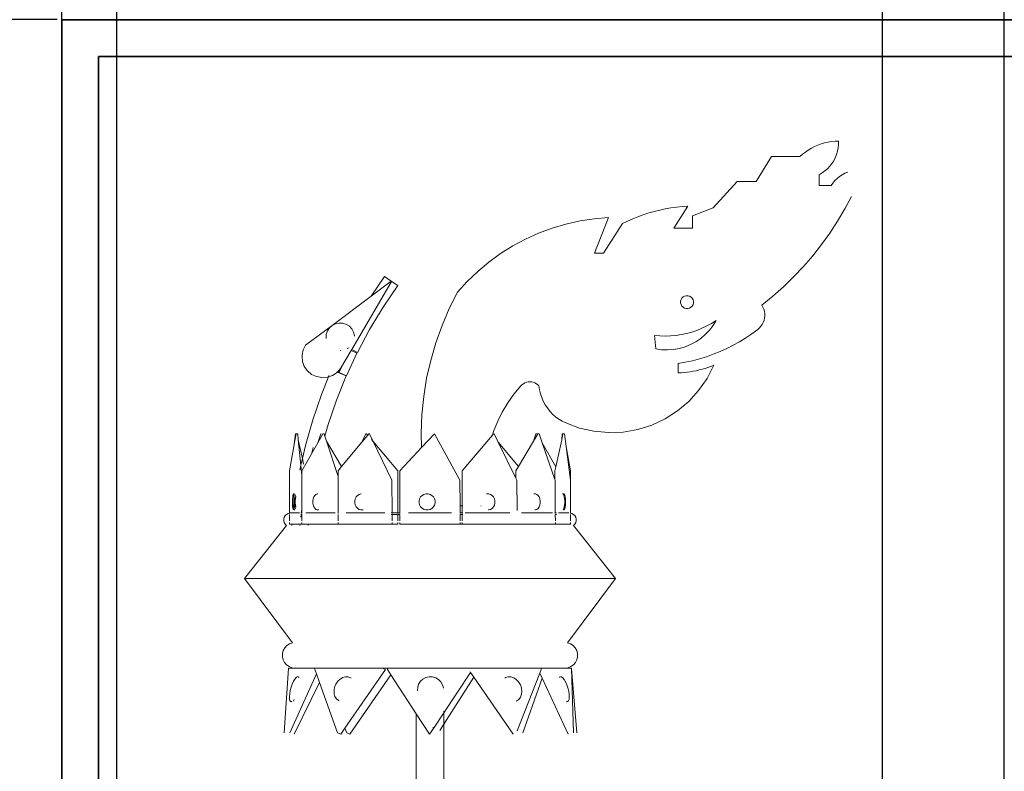
# Model space of a CAD drawing. Units: millimetres. Extents: x 446512 to 447461, y 70395 to 70610.
# Tile 12 of 39: x 446686 to 446699.43, y 70483.13 to 70493.38. Entities that reach past the tile are written whole.
import ezdxf

# ---------------------------------------------------------------- set-up
doc = ezdxf.new("R2010")
doc.units = ezdxf.units.MM
for name, color, linetype, lineweight in [('A-ANNO-DIMS', 2, 'Continuous', 18), ('A-CONS', 9, 'Continuous', 13), ('A-FURN', 7, 'Continuous', 35), ('A-FURN-DECO', 8, 'Continuous', 13)]:
    doc.layers.add(name, color=color, linetype=linetype, lineweight=lineweight)
doc.styles.get("Standard").update_dxf_attribs({"font": 'arial.ttf'})
doc.dimstyles.get("Standard").update_dxf_attribs({"dimtxt": 0.18, "dimasz": 0.18, "dimexe": 0.18, "dimexo": 0.0625, "dimgap": 0.09, "dimtad": 0, "dimtih": 1, "dimtoh": 1, "dimdec": 4, "dimzin": 0, "dimdsep": 46, "dimtxsty": 'Standard', "dimcen": 0.09, "dimadec": 0, "dimazin": 0, "dimtfac": 1, "dimtdec": 4, "dimtofl": 0, "dimtmove": 0, "dimatfit": 3, "dimfxl": 1, "dimtolj": 1, "dimtzin": 0, "dimarcsym": 0})

# ---------------------------------------------------------------- blocks, each defined once
blk = doc.blocks.new('*D21')
at = {"layer": 'A-ANNO-DIMS', "color": 0, "lineweight": -2, "transparency": 16777216}
for p, q in [((446686.51, 70493.382), (446678.043, 70493.382)), ((446678.223, 70493.202), (446678.223, 70483.563)), ((446678.223, 70473.562), (446678.223, 70483.2)), ((446686.51, 70473.382), (446678.043, 70473.382))]:
    blk.add_line(p, q, dxfattribs=at)
at = {"layer": 'A-ANNO-DIMS', "color": 0, "transparency": 16777216}
for points in [[(446678.193, 70493.202), (446678.253, 70493.202), (446678.223, 70493.382)], [(446678.193, 70473.562), (446678.253, 70473.562), (446678.223, 70473.382)]]:
    blk.add_solid(points, dxfattribs=at)
at = {"layer": 'Defpoints', "color": 0, "transparency": 16777216}
for p in [(446678.223, 70493.382), (446686.573, 70493.382), (446686.573, 70473.382)]:
    blk.add_point(p, dxfattribs=at)
at = {"layer": 'A-ANNO-DIMS', "color": 0, "transparency": 16777216, "insert": (446678.223, 70483.382), "char_height": 0.18, "attachment_point": 5}
blk.add_mtext('\\A1;20', dxfattribs=at)
blk = doc.blocks.new('*D37')
at = {"layer": 'A-ANNO-DIMS', "color": 0, "lineweight": -2, "transparency": 16777216}
for p, q in [((446686.572846, 70433.44405), (446686.572846, 70578.17492)), ((446687.323552, 70428.838404), (446687.323552, 70578.17492)), ((446686.392846, 70577.99492), (446686.212846, 70577.99492)), ((446687.503552, 70577.99492), (446687.683552, 70577.99492))]:
    blk.add_line(p, q, dxfattribs=at)
at = {"layer": 'A-ANNO-DIMS', "color": 0, "transparency": 16777216}
for points in [[(446686.392846, 70578.02492), (446686.392846, 70577.96492), (446686.572846, 70577.99492)], [(446687.503552, 70578.02492), (446687.503552, 70577.96492), (446687.323552, 70577.99492)]]:
    blk.add_solid(points, dxfattribs=at)
at = {"layer": 'Defpoints', "color": 0, "transparency": 16777216}
for p in [(446687.323552, 70577.99492), (446686.572846, 70433.38155), (446687.323552, 70428.775904)]:
    blk.add_point(p, dxfattribs=at)
at = {"layer": 'A-ANNO-DIMS', "color": 0, "transparency": 16777216, "insert": (446686.948199, 70577.99492), "char_height": 0.18, "attachment_point": 5}
blk.add_mtext('\\A1;0.75', dxfattribs=at)
blk = doc.blocks.new('*D38')
at = {"layer": 'A-ANNO-DIMS', "color": 0, "lineweight": -2, "transparency": 16777216}
for p, q in [((446687.323552, 70428.838404), (446687.323552, 70578.17492)), ((446697.765686, 70428.838404), (446697.765686, 70578.17492)), ((446687.503552, 70577.99492), (446692.090383, 70577.99492)), ((446697.585686, 70577.99492), (446692.998855, 70577.99492))]:
    blk.add_line(p, q, dxfattribs=at)
at = {"layer": 'A-ANNO-DIMS', "color": 0, "transparency": 16777216}
for points in [[(446687.503552, 70578.02492), (446687.503552, 70577.96492), (446687.323552, 70577.99492)], [(446697.585686, 70578.02492), (446697.585686, 70577.96492), (446697.765686, 70577.99492)]]:
    blk.add_solid(points, dxfattribs=at)
at = {"layer": 'Defpoints', "color": 0, "transparency": 16777216}
for p in [(446697.765686, 70577.99492), (446687.323552, 70428.775904), (446697.765686, 70428.775904)]:
    blk.add_point(p, dxfattribs=at)
at = {"layer": 'A-ANNO-DIMS', "color": 0, "transparency": 16777216, "insert": (446692.544619, 70577.99492), "char_height": 0.18, "attachment_point": 5}
blk.add_mtext('\\A1;10.442', dxfattribs=at)
blk = doc.blocks.new('*D39')
at = {"layer": 'A-ANNO-DIMS', "color": 0, "lineweight": -2, "transparency": 16777216}
for p, q in [((446697.766, 70428.838), (446697.766, 70578.175)), ((446699.429, 70433.444), (446699.429, 70578.175)), ((446697.946, 70577.995), (446698.212, 70577.995)), ((446699.249, 70577.995), (446698.982, 70577.995))]:
    blk.add_line(p, q, dxfattribs=at)
at = {"layer": 'A-ANNO-DIMS', "color": 0, "transparency": 16777216}
for points in [[(446697.946, 70578.025), (446697.946, 70577.965), (446697.766, 70577.995)], [(446699.249, 70578.025), (446699.249, 70577.965), (446699.429, 70577.995)]]:
    blk.add_solid(points, dxfattribs=at)
at = {"layer": 'Defpoints', "color": 0, "transparency": 16777216}
for p in [(446699.429, 70577.995), (446699.429, 70433.382), (446697.766, 70428.776)]:
    blk.add_point(p, dxfattribs=at)
at = {"layer": 'A-ANNO-DIMS', "color": 0, "transparency": 16777216, "insert": (446698.597, 70577.995), "char_height": 0.18, "attachment_point": 5}
blk.add_mtext('\\A1;1.663', dxfattribs=at)

msp = doc.modelspace()

# ---------------------------------------------------------------- linework, layer by layer
at = {"layer": 'A-CONS'}
msp.add_point((446686.5728, 70493.3815), dxfattribs=at)
at = {"layer": 'A-FURN'}
for p, q in [((446686.5728, 70493.3815), (446746.5728, 70493.3815)), ((446686.5728, 70473.3815), (446686.5728, 70493.3815))]:
    msp.add_line(p, q, dxfattribs=at)
for points in [[(446686.5728, 70493.3815), (446729.0084, 70493.3815), (446729.0084, 70473.3815), (446686.5728, 70473.3815)], [(446687.0728, 70492.8815), (446728.5084, 70492.8815), (446728.5084, 70473.8815), (446687.0728, 70473.8815)]]:
    msp.add_lwpolyline(points, close=True, dxfattribs=at)
at = {"layer": 'A-FURN-DECO'}
for p, q in [((446696.7153, 70491.5764), (446696.7552, 70491.6041)), ((446696.7552, 70491.6041), (446696.7968, 70491.6292)), ((446696.7968, 70491.6292), (446696.84, 70491.6515)), ((446696.84, 70491.6515), (446696.8844, 70491.6711)), ((446696.8844, 70491.6711), (446696.9301, 70491.6877)), ((446696.9301, 70491.6877), (446696.9767, 70491.7015)), ((446696.9767, 70491.7015), (446697.024, 70491.7122)), ((446697.024, 70491.7122), (446697.072, 70491.7198)), ((446697.072, 70491.7198), (446697.1204, 70491.7244)), ((446697.1204, 70491.7244), (446697.1689, 70491.7259)), ((446697.1638, 70491.6329), (446697.1547, 70491.5872)), ((446697.1686, 70491.6793), (446697.1638, 70491.6329)), ((446697.1689, 70491.7259), (446697.1686, 70491.6793)), ((446696.0452, 70491.1756), (446696.2545, 70491.5137)), ((446696.2545, 70491.5137), (446696.6411, 70491.5137)), ((446696.6411, 70491.5137), (446696.6772, 70491.5463)), ((446696.6772, 70491.5463), (446696.7153, 70491.5764)), ((446697.1237, 70491.4993), (446697.1021, 70491.458)), ((446697.1413, 70491.5425), (446697.1237, 70491.4993)), ((446697.1547, 70491.5872), (446697.1413, 70491.5425)), ((446697.0155, 70491.3487), (446696.9802, 70491.3182)), ((446697.0478, 70491.3823), (446697.0155, 70491.3487)), ((446697.0767, 70491.4189), (446697.0478, 70491.3823)), ((446697.1021, 70491.458), (446697.0767, 70491.4189)), ((446696.9421, 70491.2912), (446696.9017, 70491.268)), ((446696.9017, 70491.268), (446696.9017, 70491.1188)), ((446696.9802, 70491.3182), (446696.9421, 70491.2912)), ((446697.118, 70491.1867), (446697.148, 70491.2166)), ((446697.148, 70491.2166), (446697.1808, 70491.2435)), ((446697.1808, 70491.2435), (446697.2159, 70491.2671)), ((446697.2159, 70491.2671), (446697.2532, 70491.2872)), ((446697.2532, 70491.2872), (446697.2923, 70491.3036)), ((446695.4573, 70490.8173), (446695.7856, 70491.1756)), ((446695.7856, 70491.1756), (446696.0452, 70491.1756)), ((446696.9017, 70491.1188), (446697.0674, 70491.1188)), ((446697.0674, 70491.1188), (446697.0911, 70491.154)), ((446697.0911, 70491.154), (446697.118, 70491.1867)), ((446697.3425, 70490.9725), (446697.2517, 70490.8013)), ((446694.7284, 70490.7852), (446694.8042, 70490.801)), ((446694.8042, 70490.801), (446694.8805, 70490.8141)), ((446694.8805, 70490.8141), (446694.9573, 70490.8245)), ((446695.1116, 70490.8369), (446694.921, 70490.5393)), ((446694.9573, 70490.8245), (446695.0343, 70490.8321)), ((446695.0343, 70490.8321), (446695.1116, 70490.8369)), ((446695.175, 70490.705), (446695.4573, 70490.8173)), ((446697.2517, 70490.8013), (446697.1532, 70490.6345)), ((446693.6414, 70490.6372), (446693.836, 70490.6671)), ((446693.836, 70490.6671), (446694.0321, 70490.6837)), ((446694.0321, 70490.6837), (446693.8395, 70490.1957)), ((446694.2897, 70490.6344), (446694.3604, 70490.666)), ((446694.3604, 70490.666), (446694.4322, 70490.6951)), ((446694.4322, 70490.6951), (446694.505, 70490.7216)), ((446694.505, 70490.7216), (446694.5787, 70490.7454)), ((446694.5787, 70490.7454), (446694.6532, 70490.7666)), ((446694.6532, 70490.7666), (446694.7284, 70490.7852)), ((446695.175, 70490.5393), (446695.175, 70490.705)), ((446693.0762, 70490.4696), (446693.2607, 70490.5382)), ((446693.2607, 70490.5382), (446693.4494, 70490.5942)), ((446693.4494, 70490.5942), (446693.6414, 70490.6372)), ((446693.961, 70490.1957), (446694.2202, 70490.6003)), ((446694.2202, 70490.6003), (446694.2897, 70490.6344)), ((446694.921, 70490.5393), (446695.175, 70490.5393)), ((446697.1532, 70490.6345), (446697.0475, 70490.4721)), ((446692.8968, 70490.3885), (446693.0762, 70490.4696)), ((446697.0475, 70490.4721), (446696.9346, 70490.3147)), ((446692.5566, 70490.1909), (446692.7233, 70490.2955)), ((446692.7233, 70490.2955), (446692.8968, 70490.3885)), ((446696.9346, 70490.3147), (446696.8148, 70490.1624)), ((446692.3973, 70490.0753), (446692.5566, 70490.1909)), ((446693.8395, 70490.1957), (446693.961, 70490.1957)), ((446696.8148, 70490.1624), (446696.6883, 70490.0156)), ((446692.2463, 70489.9491), (446692.3973, 70490.0753)), ((446696.6883, 70490.0156), (446696.5554, 70489.8746)), ((446690.9762, 70489.8801), (446690.7926, 70489.6121)), ((446691.0674, 70489.8177), (446690.9762, 70489.8801)), ((446692.1042, 70489.8129), (446692.2463, 70489.9491)), ((446696.5554, 70489.8746), (446696.4164, 70489.7397)), ((446691.0674, 70489.8034), (446690.5277, 70488.8832)), ((446691.0674, 70489.8177), (446690.7926, 70489.6121)), ((446690.9564, 70489.4602), (446691.1585, 70489.7553)), ((446691.0674, 70489.8034), (446691.0674, 70489.8177)), ((446691.1585, 70489.7553), (446691.0674, 70489.8177)), ((446691.9716, 70489.6674), (446692.1042, 70489.8129)), ((446696.4164, 70489.7397), (446696.2714, 70489.6111)), ((446690.7926, 70489.6121), (446690.2614, 70489.2121)), ((446691.9716, 70489.6674), (446691.8583, 70489.4434)), ((446695.0198, 70489.5639), (446695.0314, 70489.5838)), ((446695.0314, 70489.5838), (446695.0478, 70489.6001)), ((446695.0478, 70489.6001), (446695.0679, 70489.6115)), ((446695.0679, 70489.6115), (446695.0902, 70489.6174)), ((446695.0902, 70489.6174), (446695.1133, 70489.6172)), ((446695.1133, 70489.6172), (446695.1355, 70489.6112)), ((446695.1355, 70489.6112), (446695.1554, 70489.5995)), ((446695.1554, 70489.5995), (446695.1717, 70489.5831)), ((446696.2714, 70489.6111), (446696.1209, 70489.4891)), ((446690.772, 70489.1572), (446690.9564, 70489.4602)), ((446695.0136, 70489.5186), (446695.0137, 70489.5417)), ((446695.0195, 70489.4963), (446695.0136, 70489.5186)), ((446695.0137, 70489.5417), (446695.0198, 70489.5639)), ((446695.0309, 70489.4763), (446695.0195, 70489.4963)), ((446695.0471, 70489.4599), (446695.0309, 70489.4763)), ((446695.067, 70489.4482), (446695.0471, 70489.4599)), ((446695.1547, 70489.4593), (446695.1347, 70489.4479)), ((446695.1711, 70489.4755), (446695.1547, 70489.4593)), ((446695.1827, 70489.4954), (446695.1711, 70489.4755)), ((446695.1717, 70489.5831), (446695.1831, 70489.5631)), ((446695.1888, 70489.5177), (446695.1827, 70489.4954)), ((446695.1831, 70489.5631), (446695.1889, 70489.5408)), ((446695.1889, 70489.5408), (446695.1888, 70489.5177)), ((446696.1209, 70489.4891), (446696.1363, 70489.4624)), ((446696.1363, 70489.4624), (446696.1482, 70489.4339)), ((446691.8583, 70489.4434), (446691.7591, 70489.2129)), ((446695.0893, 70489.4421), (446695.067, 70489.4482)), ((446695.1124, 70489.442), (446695.0893, 70489.4421)), ((446695.1347, 70489.4479), (446695.1124, 70489.442)), ((446696.1482, 70489.4339), (446696.1565, 70489.4042)), ((446696.1565, 70489.4042), (446696.161, 70489.3736)), ((446696.1617, 70489.3428), (446696.1586, 70489.3121)), ((446696.161, 70489.3736), (446696.1617, 70489.3428)), ((446690.2614, 70489.2121), (446689.8973, 70488.9421)), ((446690.2238, 70489.1795), (446690.2614, 70489.2121)), ((446690.2614, 70489.2121), (446690.3063, 70489.2342)), ((446690.3063, 70489.2342), (446690.3557, 70489.2444)), ((446690.3557, 70489.2444), (446690.4061, 70489.2418)), ((446690.4061, 70489.2418), (446690.4541, 70489.2267)), ((446690.4541, 70489.2267), (446690.4964, 70489.2002)), ((446690.4964, 70489.2002), (446690.5301, 70489.1639)), ((446691.7591, 70489.2129), (446691.6743, 70488.9767)), ((446695.3717, 70489.2046), (446695.3051, 70489.1729)), ((446695.4363, 70489.2402), (446695.3717, 70489.2046)), ((446695.4562, 70489.2103), (446695.4067, 70489.1459)), ((446695.4988, 70489.2795), (446695.4363, 70489.2402)), ((446695.4988, 70489.2795), (446695.4562, 70489.2103)), ((446696.1092, 70489.2002), (446696.0887, 70489.1771)), ((446696.1267, 70489.2256), (446696.1092, 70489.2002)), ((446696.1409, 70489.253), (446696.1267, 70489.2256)), ((446696.1516, 70489.282), (446696.1409, 70489.253)), ((446696.1586, 70489.3121), (446696.1516, 70489.282)), ((446690.1781, 70489.0436), (446690.1807, 70489.0923)), ((446690.1807, 70489.0923), (446690.1964, 70489.1387)), ((446690.1964, 70489.1387), (446690.2238, 70489.1795)), ((446690.5301, 70489.1639), (446690.553, 70489.1205)), ((446690.553, 70489.1205), (446690.5635, 70489.0728)), ((446690.5631, 70489.0659), (446690.5635, 70489.0728)), ((446690.5631, 70489.0659), (446690.5635, 70489.0642)), ((446690.772, 70489.1572), (446690.6043, 70488.8447)), ((446694.7296, 70489.0686), (446694.6561, 70489.0749)), ((446694.6561, 70489.0749), (446694.6742, 70488.8914)), ((446694.8034, 70489.0666), (446694.7296, 70489.0686)), ((446694.8771, 70489.069), (446694.8034, 70489.0666)), ((446694.9506, 70489.0757), (446694.8771, 70489.069)), ((446695.0235, 70489.0868), (446694.9506, 70489.0757)), ((446695.0957, 70489.102), (446695.0235, 70489.0868)), ((446695.1668, 70489.1215), (446695.0957, 70489.102)), ((446695.2367, 70489.1452), (446695.1668, 70489.1215)), ((446695.3051, 70489.1729), (446695.2367, 70489.1452)), ((446695.3506, 70489.0872), (446695.2887, 70489.0346)), ((446695.4067, 70489.1459), (446695.3506, 70489.0872)), ((446695.9853, 70489.0978), (446695.9028, 70489.0422)), ((446696.0655, 70489.1568), (446695.9853, 70489.0978)), ((446696.0887, 70489.1771), (446696.0655, 70489.1568)), ((446689.8973, 70488.9421), (446689.8648, 70488.8771)), ((446690.1785, 70489.0419), (446690.1781, 70489.0436)), ((446690.1781, 70489.035), (446690.1785, 70489.0419)), ((446691.6743, 70488.9767), (446691.6043, 70488.7356)), ((446695.0748, 70488.9198), (446694.9968, 70488.8973)), ((446695.15, 70488.9505), (446695.0748, 70488.9198)), ((446695.2216, 70488.9889), (446695.15, 70488.9505)), ((446695.2887, 70489.0346), (446695.2216, 70488.9889)), ((446695.731, 70488.9416), (446695.6421, 70488.8968)), ((446695.8179, 70488.9901), (446695.731, 70488.9416)), ((446695.9028, 70489.0422), (446695.8179, 70488.9901)), ((446689.8648, 70488.8771), (446689.8508, 70488.8062)), ((446689.8508, 70488.7919), (446689.8508, 70488.8062)), ((446689.8508, 70488.7919), (446689.8563, 70488.7199)), ((446690.3735, 70488.8727), (446690.3696, 70488.8643)), ((446690.52, 70488.8701), (446690.3759, 70488.6244)), ((446690.4548, 70488.5258), (446690.5989, 70488.8331)), ((446690.464, 70488.8963), (446690.473, 70488.8922)), ((446690.4885, 70488.9029), (446690.4822, 70488.906)), ((446690.5277, 70488.8832), (446690.52, 70488.8701)), ((446690.5989, 70488.8331), (446690.52, 70488.8701)), ((446690.5277, 70488.8832), (446690.6043, 70488.8447)), ((446694.7547, 70488.8801), (446694.6742, 70488.8914)), ((446694.8358, 70488.8773), (446694.7547, 70488.8801)), ((446694.9168, 70488.883), (446694.8358, 70488.8773)), ((446694.9968, 70488.8973), (446694.9168, 70488.883)), ((446695.3653, 70488.7853), (446695.2702, 70488.756)), ((446695.4591, 70488.8186), (446695.3653, 70488.7853)), ((446695.5515, 70488.8558), (446695.4591, 70488.8186)), ((446695.6421, 70488.8968), (446695.5515, 70488.8558)), ((446689.8563, 70488.7199), (446689.8809, 70488.6518)), ((446689.8809, 70488.6518), (446689.923, 70488.5921)), ((446690.3917, 70488.6514), (446690.3548, 70488.5727)), ((446691.6043, 70488.7356), (446691.5493, 70488.4908)), ((446695.0767, 70488.7094), (446694.9787, 70488.6923)), ((446694.9787, 70488.6923), (446694.9787, 70488.5652)), ((446695.174, 70488.7307), (446695.0767, 70488.7094)), ((446695.2702, 70488.756), (446695.174, 70488.7307)), ((446695.4649, 70488.6683), (446695.3736, 70488.4897)), ((446695.3869, 70488.6393), (446695.4261, 70488.6532)), ((446695.4261, 70488.6532), (446695.4649, 70488.6683)), ((446689.923, 70488.5921), (446689.9796, 70488.545)), ((446689.9796, 70488.545), (446690.0468, 70488.5136)), ((446690.0468, 70488.5136), (446690.1203, 70488.5001)), ((446690.2103, 70488.5106), (446690.1138, 70488.2721)), ((446690.1948, 70488.5054), (446690.2103, 70488.5106)), ((446690.2103, 70488.5106), (446690.2653, 70488.5292)), ((446690.2169, 70488.5272), (446690.2103, 70488.5106)), ((446690.2653, 70488.5292), (446690.3271, 70488.5698)), ((446690.3208, 70488.1948), (446690.4538, 70488.5236)), ((446690.3223, 70488.5809), (446690.3329, 70488.5763)), ((446690.3271, 70488.5698), (446690.3329, 70488.5763)), ((446690.3371, 70488.581), (446690.3289, 70488.5848)), ((446690.3329, 70488.5763), (446690.3371, 70488.581)), ((446690.3329, 70488.5763), (446690.4538, 70488.5236)), ((446690.3371, 70488.581), (446690.3759, 70488.6244)), ((446690.3371, 70488.581), (446690.4548, 70488.5258)), ((446690.3548, 70488.5727), (446690.3525, 70488.5678)), ((446694.9787, 70488.5652), (446695.0203, 70488.5672)), ((446695.0203, 70488.5672), (446695.0618, 70488.5703)), ((446695.0618, 70488.5703), (446695.1032, 70488.5747)), ((446695.1032, 70488.5747), (446695.1445, 70488.5803)), ((446695.1445, 70488.5803), (446695.1855, 70488.5871)), ((446695.1855, 70488.5871), (446695.2264, 70488.5952)), ((446695.2264, 70488.5952), (446695.267, 70488.6044)), ((446695.267, 70488.6044), (446695.3073, 70488.6149)), ((446695.3073, 70488.6149), (446695.3473, 70488.6265)), ((446695.3473, 70488.6265), (446695.3869, 70488.6393)), ((446690.1203, 70488.5001), (446690.1948, 70488.5054)), ((446691.5493, 70488.4908), (446691.5095, 70488.2429)), ((446692.8329, 70488.3878), (446692.7393, 70488.2755)), ((446692.8497, 70488.4039), (446692.8329, 70488.3878)), ((446692.8685, 70488.4176), (446692.8497, 70488.4039)), ((446692.8891, 70488.4286), (446692.8685, 70488.4176)), ((446692.9111, 70488.4365), (446692.8891, 70488.4286)), ((446692.9339, 70488.4414), (446692.9111, 70488.4365)), ((446692.9571, 70488.443), (446692.9339, 70488.4414)), ((446692.9804, 70488.4414), (446692.9571, 70488.443)), ((446693.0032, 70488.4365), (446692.9804, 70488.4414)), ((446693.0251, 70488.4286), (446693.0032, 70488.4365)), ((446693.0457, 70488.4176), (446693.0251, 70488.4286)), ((446693.0646, 70488.4039), (446693.0457, 70488.4176)), ((446693.0814, 70488.3878), (446693.0646, 70488.4039)), ((446693.0894, 70488.3339), (446693.0814, 70488.3878)), ((446695.3736, 70488.4897), (446695.2594, 70488.3247)), ((446690.1138, 70488.2721), (446689.9949, 70487.9253)), ((446691.5095, 70488.2429), (446691.4851, 70487.9931)), ((446692.7393, 70488.2755), (446692.6548, 70488.1561)), ((446693.1021, 70488.281), (446693.0894, 70488.3339)), ((446693.1193, 70488.2293), (446693.1021, 70488.281)), ((446695.2594, 70488.3247), (446695.1246, 70488.1761)), ((446690.2058, 70487.8593), (446690.3208, 70488.1948)), ((446692.6548, 70488.1561), (446692.58, 70488.0305)), ((446693.141, 70488.1794), (446693.1193, 70488.2293)), ((446693.1669, 70488.1315), (446693.141, 70488.1794)), ((446693.1969, 70488.0861), (446693.1669, 70488.1315)), ((446695.1246, 70488.1761), (446694.9714, 70488.0466)), ((446691.4851, 70487.9931), (446691.4762, 70487.7423)), ((446692.58, 70488.0305), (446692.5154, 70487.8993)), ((446693.2308, 70488.0435), (446693.1969, 70488.0861)), ((446693.2682, 70488.0039), (446693.2308, 70488.0435)), ((446693.3089, 70487.9678), (446693.2682, 70488.0039)), ((446694.9714, 70488.0466), (446694.8024, 70487.9384)), ((446689.9949, 70487.9253), (446689.8949, 70487.5726)), ((446690.1611, 70487.7015), (446690.2058, 70487.8593)), ((446692.5154, 70487.8993), (446692.4613, 70487.7635)), ((446693.3526, 70487.9353), (446693.3089, 70487.9678)), ((446693.399, 70487.9068), (446693.3526, 70487.9353)), ((446693.4476, 70487.8824), (446693.399, 70487.9068)), ((446693.6358, 70487.8127), (446693.4476, 70487.8824)), ((446694.6207, 70487.8534), (446694.4293, 70487.7931)), ((446694.8024, 70487.9384), (446694.6207, 70487.8534)), ((446689.7422, 70487.5943), (446689.7597, 70487.732)), ((446689.7686, 70487.732), (446689.7422, 70487.5943)), ((446689.7686, 70487.732), (446689.7597, 70487.732)), ((446689.7686, 70487.732), (446689.7903, 70487.732)), ((446689.7985, 70487.653), (446689.7903, 70487.732)), ((446690.0658, 70487.6129), (446690.1072, 70487.732)), ((446690.1333, 70487.732), (446690.0658, 70487.6129)), ((446690.1123, 70487.732), (446690.1072, 70487.732)), ((446690.151, 70487.732), (446690.1333, 70487.732)), ((446690.1611, 70487.7015), (446690.151, 70487.732)), ((446690.6667, 70487.6207), (446690.7216, 70487.732)), ((446690.7455, 70487.7153), (446690.6667, 70487.6207)), ((446690.7312, 70487.732), (446690.7216, 70487.732)), ((446690.7312, 70487.732), (446690.7455, 70487.7153)), ((446690.7594, 70487.732), (446690.7455, 70487.7153)), ((446690.7699, 70487.732), (446690.7594, 70487.732)), ((446690.8204, 70487.6273), (446690.7699, 70487.732)), ((446691.4762, 70487.7423), (446691.4814, 70487.5462)), ((446691.6572, 70487.732), (446691.4814, 70487.5462)), ((446692.0025, 70487.1025), (446691.6572, 70487.732)), ((446692.446, 70487.714), (446692.0321, 70487.2307)), ((446692.446, 70487.714), (446692.4417, 70487.7003)), ((446692.4472, 70487.7181), (446692.446, 70487.714)), ((446692.446, 70487.714), (446692.4496, 70487.7096)), ((446692.4613, 70487.7635), (446692.4472, 70487.7181)), ((446692.4591, 70487.732), (446692.4472, 70487.7181)), ((446692.4591, 70487.732), (446692.4687, 70487.732)), ((446692.5236, 70487.6207), (446692.4687, 70487.732)), ((446693.0069, 70487.6333), (446693.0393, 70487.732)), ((446693.0614, 70487.7242), (446693.0069, 70487.6333)), ((446693.0393, 70487.732), (446693.057, 70487.732)), ((446693.057, 70487.732), (446693.0614, 70487.7242)), ((446693.0661, 70487.732), (446693.0614, 70487.7242)), ((446693.0661, 70487.732), (446693.0831, 70487.732)), ((446693.1245, 70487.6129), (446693.0831, 70487.732)), ((446693.3918, 70487.653), (446693.4, 70487.732)), ((446693.4091, 70487.732), (446693.3918, 70487.653)), ((446693.4, 70487.732), (446693.4091, 70487.732)), ((446693.4091, 70487.732), (446693.4306, 70487.732)), ((446693.4306, 70487.732), (446693.4525, 70487.5599)), ((446693.8314, 70487.7684), (446693.6358, 70487.8127)), ((446694.0312, 70487.7502), (446693.8314, 70487.7684)), ((446694.2317, 70487.7585), (446694.0312, 70487.7502)), ((446694.4293, 70487.7931), (446694.2317, 70487.7585)), ((446689.7378, 70487.5599), (446689.7422, 70487.5943)), ((446689.7985, 70487.653), (446689.855, 70487.3957)), ((446689.8346, 70487.3054), (446689.7985, 70487.653)), ((446690.0658, 70487.6129), (446689.849, 70487.2307)), ((446689.8949, 70487.5726), (446689.855, 70487.3957)), ((446690.1834, 70487.6333), (446690.1611, 70487.7015)), ((446690.1834, 70487.6333), (446690.3901, 70487.2886)), ((446690.3419, 70487.1511), (446690.1834, 70487.6333)), ((446690.6667, 70487.6207), (446690.3901, 70487.2886)), ((446690.7961, 70487.6558), (446690.8204, 70487.6273)), ((446690.8204, 70487.6273), (446691.1582, 70487.2307)), ((446691.0736, 70487.1025), (446690.8204, 70487.6273)), ((446692.5236, 70487.6207), (446692.8002, 70487.2886)), ((446692.5236, 70487.6207), (446692.7654, 70487.1306)), ((446693.0069, 70487.6333), (446692.8002, 70487.2886)), ((446693.1245, 70487.6129), (446693.3109, 70487.2842)), ((446693.1245, 70487.6129), (446693.2991, 70487.1102)), ((446693.3918, 70487.653), (446693.3109, 70487.2842)), ((446689.7378, 70487.5599), (446689.6789, 70487.2307)), ((446690.002, 70487.5453), (446689.9851, 70487.4707)), ((446691.4814, 70487.5462), (446691.1826, 70487.2307)), ((446693.4525, 70487.5599), (446693.5114, 70487.2307)), ((446693.5107, 70487.1025), (446693.4525, 70487.5599)), ((446689.8346, 70487.3054), (446689.8197, 70487.2395)), ((446689.855, 70487.3957), (446689.8346, 70487.3054)), ((446689.849, 70487.1659), (446689.8346, 70487.3054)), ((446689.855, 70487.3957), (446689.8713, 70487.3212)), ((446689.6789, 70487.2307), (446689.6807, 70487.1103)), ((446689.849, 70487.2307), (446689.849, 70487.1659)), ((446690.3901, 70487.2886), (446690.3419, 70487.2307)), ((446690.3419, 70487.2307), (446690.3419, 70487.1511)), ((446691.1582, 70487.2307), (446691.1582, 70486.6542)), ((446691.1826, 70487.2307), (446691.1826, 70486.6542)), ((446692.0321, 70487.2307), (446692.0321, 70486.7516)), ((446692.8002, 70487.2886), (446692.7654, 70487.2307)), ((446692.7654, 70487.2307), (446692.7654, 70487.1306)), ((446693.3109, 70487.2842), (446693.2991, 70487.2307)), ((446693.2991, 70487.2307), (446693.2991, 70487.1102)), ((446693.5114, 70487.2307), (446693.5107, 70487.1025)), ((446689.6797, 70487.1025), (446689.6788, 70486.6528)), ((446689.6797, 70487.1025), (446689.6807, 70487.1103)), ((446689.849, 70487.1659), (446689.849, 70486.6542)), ((446690.3419, 70487.1511), (446690.3419, 70486.648)), ((446691.0736, 70487.1025), (446691.077, 70486.6542)), ((446692.0025, 70487.1025), (446692.0055, 70486.7514)), ((446692.7793, 70487.1025), (446692.7654, 70487.1306)), ((446692.7793, 70487.1025), (446692.7825, 70486.6881)), ((446693.3018, 70487.1025), (446693.2991, 70487.1102)), ((446693.3018, 70487.1025), (446693.3043, 70486.6542)), ((446693.5107, 70487.1025), (446693.5115, 70486.6528)), ((446689.7257, 70486.8933), (446689.7305, 70486.9077)), ((446689.7305, 70486.9077), (446689.7357, 70486.915)), ((446689.7466, 70486.915), (446689.7357, 70486.915)), ((446689.7366, 70486.8933), (446689.7413, 70486.9077)), ((446689.7413, 70486.9077), (446689.7466, 70486.915)), ((446689.7598, 70486.8998), (446689.757, 70486.8929)), ((446689.7604, 70486.898), (446689.757, 70486.8929)), ((446690.023, 70486.8933), (446690.038, 70486.9077)), ((446690.038, 70486.9077), (446690.0547, 70486.915)), ((446690.0635, 70486.915), (446690.0547, 70486.915)), ((446690.605, 70486.8933), (446690.627, 70486.9077)), ((446690.627, 70486.9077), (446690.6516, 70486.915)), ((446690.6568, 70486.915), (446690.6516, 70486.915)), ((446691.4878, 70486.8933), (446691.5128, 70486.9077)), ((446691.5128, 70486.9077), (446691.5407, 70486.915)), ((446691.5407, 70486.915), (446691.5695, 70486.915)), ((446691.5695, 70486.915), (446691.5973, 70486.9074)), ((446691.5973, 70486.9074), (446691.6223, 70486.8929)), ((446692.3638, 70486.915), (446692.3687, 70486.915)), ((446692.3687, 70486.915), (446692.3946, 70486.915)), ((446692.3946, 70486.915), (446692.4196, 70486.9074)), ((446692.4196, 70486.9074), (446692.4421, 70486.8929)), ((446693.0093, 70486.915), (446693.0179, 70486.915)), ((446693.0179, 70486.915), (446693.0361, 70486.915)), ((446693.0361, 70486.915), (446693.0537, 70486.9074)), ((446693.0537, 70486.9074), (446693.0695, 70486.8929)), ((446693.4036, 70486.915), (446693.4103, 70486.915)), ((446693.4103, 70486.915), (446693.4167, 70486.9074)), ((446693.4103, 70486.915), (446693.4144, 70486.915)), ((446693.4144, 70486.915), (446693.421, 70486.915)), ((446693.4167, 70486.9074), (446693.4225, 70486.8929)), ((446693.421, 70486.915), (446693.4275, 70486.9074)), ((446693.4275, 70486.9074), (446693.4333, 70486.8929)), ((446689.7177, 70486.8202), (446689.7191, 70486.848)), ((446689.7177, 70486.7914), (446689.7177, 70486.8202)), ((446689.7191, 70486.7635), (446689.7177, 70486.7914)), ((446689.7191, 70486.848), (446689.7219, 70486.873)), ((446689.7218, 70486.7385), (446689.7191, 70486.7635)), ((446689.7219, 70486.873), (446689.7257, 70486.8933)), ((446689.7285, 70486.8202), (446689.73, 70486.848)), ((446689.7285, 70486.7914), (446689.7285, 70486.8202)), ((446689.7299, 70486.7635), (446689.7285, 70486.7914)), ((446689.7326, 70486.7385), (446689.7299, 70486.7635)), ((446689.73, 70486.848), (446689.7327, 70486.873)), ((446689.7327, 70486.873), (446689.7366, 70486.8933)), ((446689.7473, 70486.7908), (446689.7365, 70486.718)), ((446689.749, 70486.8475), (446689.7473, 70486.8196)), ((446689.7473, 70486.8196), (446689.7473, 70486.7908)), ((446689.7473, 70486.7908), (446689.7491, 70486.763)), ((446689.7523, 70486.8725), (446689.749, 70486.8475)), ((446689.7528, 70486.8536), (446689.749, 70486.8475)), ((446689.757, 70486.8929), (446689.7523, 70486.8725)), ((446689.7523, 70486.8725), (446689.7528, 70486.8536)), ((446689.7597, 70486.8475), (446689.758, 70486.8196)), ((446689.758, 70486.8196), (446689.7581, 70486.7908)), ((446689.7581, 70486.7908), (446689.7598, 70486.763)), ((446689.7631, 70486.8725), (446689.7597, 70486.8475)), ((446689.7646, 70486.8791), (446689.7631, 70486.8725)), ((446689.9975, 70486.8202), (446690.002, 70486.848)), ((446689.9975, 70486.7914), (446689.9975, 70486.8202)), ((446690.0019, 70486.7635), (446689.9975, 70486.7914)), ((446690.0105, 70486.7385), (446690.0019, 70486.7635)), ((446690.002, 70486.848), (446690.0107, 70486.873)), ((446690.0107, 70486.873), (446690.023, 70486.8933)), ((446690.5676, 70486.7914), (446690.5677, 70486.8202)), ((446690.5741, 70486.7635), (446690.5676, 70486.7914)), ((446690.5677, 70486.8202), (446690.5743, 70486.848)), ((446690.5867, 70486.7385), (446690.5741, 70486.7635)), ((446690.5743, 70486.848), (446690.5871, 70486.873)), ((446690.5871, 70486.873), (446690.605, 70486.8933)), ((446691.4452, 70486.7914), (446691.4453, 70486.8202)), ((446691.4526, 70486.7635), (446691.4452, 70486.7914)), ((446691.4453, 70486.8202), (446691.4528, 70486.848)), ((446691.467, 70486.7385), (446691.4526, 70486.7635)), ((446691.4528, 70486.848), (446691.4673, 70486.873)), ((446691.4673, 70486.873), (446691.4878, 70486.8933)), ((446691.6223, 70486.8929), (446691.6426, 70486.8725)), ((446691.6426, 70486.8725), (446691.6569, 70486.8475)), ((446691.6643, 70486.7908), (446691.6567, 70486.763)), ((446691.6569, 70486.8475), (446691.6643, 70486.8196)), ((446691.6643, 70486.8196), (446691.6643, 70486.7908)), ((446692.4421, 70486.8929), (446692.4604, 70486.8725)), ((446692.4604, 70486.8725), (446692.4733, 70486.8475)), ((446692.4799, 70486.7908), (446692.4731, 70486.763)), ((446692.4733, 70486.8475), (446692.4799, 70486.8196)), ((446692.4799, 70486.8196), (446692.4799, 70486.7908)), ((446693.0695, 70486.8929), (446693.0824, 70486.8725)), ((446693.0824, 70486.8725), (446693.0915, 70486.8475)), ((446693.0961, 70486.7908), (446693.0914, 70486.763)), ((446693.0915, 70486.8475), (446693.0962, 70486.8196)), ((446693.0962, 70486.8196), (446693.0961, 70486.7908)), ((446693.4225, 70486.8929), (446693.4272, 70486.8725)), ((446693.4272, 70486.8725), (446693.4306, 70486.8475)), ((446693.4323, 70486.7908), (446693.4305, 70486.763)), ((446693.4306, 70486.8475), (446693.4323, 70486.8196)), ((446693.4323, 70486.8196), (446693.4323, 70486.7908)), ((446693.4333, 70486.8929), (446693.438, 70486.8725)), ((446693.438, 70486.8725), (446693.4413, 70486.8475)), ((446693.4413, 70486.8475), (446693.443, 70486.8196)), ((446693.443, 70486.7908), (446693.4413, 70486.763)), ((446693.443, 70486.8196), (446693.443, 70486.7908)), ((446689.6198, 70486.6182), (446689.6379, 70486.6357)), ((446689.6379, 70486.6357), (446689.66, 70486.648)), ((446689.66, 70486.648), (446689.6788, 70486.6528)), ((446689.6787, 70486.6357), (446689.6785, 70486.547)), ((446689.6788, 70486.6528), (446689.6844, 70486.6542)), ((446689.6788, 70486.6528), (446689.6788, 70486.648)), ((446689.6844, 70486.6542), (446689.6887, 70486.6542)), ((446689.6844, 70486.6542), (446689.6862, 70486.6542)), ((446689.8138, 70486.6542), (446689.6887, 70486.6542)), ((446689.7256, 70486.718), (446689.7218, 70486.7385)), ((446689.7303, 70486.7036), (446689.7256, 70486.718)), ((446689.7356, 70486.696), (446689.7303, 70486.7036)), ((446689.7365, 70486.718), (446689.7326, 70486.7385)), ((446689.7411, 70486.6959), (446689.7356, 70486.696)), ((446689.7412, 70486.7036), (446689.7365, 70486.718)), ((446689.7465, 70486.696), (446689.7411, 70486.6959)), ((446689.7465, 70486.696), (446689.7412, 70486.7036)), ((446689.7519, 70486.6959), (446689.7465, 70486.696)), ((446689.7491, 70486.763), (446689.7524, 70486.738)), ((446689.7524, 70486.738), (446689.7571, 70486.7177)), ((446689.7571, 70486.7177), (446689.7598, 70486.7112)), ((446689.7598, 70486.763), (446689.7632, 70486.738)), ((446689.7632, 70486.738), (446689.7646, 70486.7318)), ((446689.849, 70486.6542), (446689.8346, 70486.6542)), ((446689.8391, 70486.6357), (446689.8347, 70486.5979)), ((446689.849, 70486.6341), (446689.8347, 70486.6341)), ((446689.849, 70486.7227), (446689.8405, 70486.648)), ((446689.849, 70486.6542), (446689.849, 70486.648)), ((446689.849, 70486.6357), (446689.849, 70486.6341)), ((446689.849, 70486.6341), (446689.849, 70486.547)), ((446690.3002, 70486.6542), (446689.9013, 70486.6542)), ((446690.0227, 70486.718), (446690.0105, 70486.7385)), ((446690.0376, 70486.7036), (446690.0227, 70486.718)), ((446690.0543, 70486.696), (446690.0376, 70486.7036)), ((446690.0716, 70486.6959), (446690.0543, 70486.696)), ((446690.0804, 70486.6959), (446690.0716, 70486.6959)), ((446690.3419, 70486.6357), (446690.3419, 70486.547)), ((446690.4496, 70486.6542), (446690.9806, 70486.6542)), ((446690.6046, 70486.718), (446690.5867, 70486.7385)), ((446690.6266, 70486.7036), (446690.6046, 70486.718)), ((446690.6511, 70486.696), (446690.6266, 70486.7036)), ((446690.6764, 70486.6959), (446690.6511, 70486.696)), ((446690.6817, 70486.6959), (446690.6764, 70486.6959)), ((446691.077, 70486.6542), (446691.0665, 70486.6542)), ((446691.0772, 70486.6341), (446691.0666, 70486.6341)), ((446691.077, 70486.6542), (446691.077, 70486.648)), ((446691.1582, 70486.6542), (446691.077, 70486.6542)), ((446691.0771, 70486.6357), (446691.0772, 70486.6341)), ((446691.0772, 70486.6341), (446691.0778, 70486.547)), ((446691.1582, 70486.6341), (446691.0772, 70486.6341)), ((446691.1582, 70486.6542), (446691.1826, 70486.6542)), ((446691.1582, 70486.6542), (446691.1582, 70486.648)), ((446691.1582, 70486.6357), (446691.1582, 70486.6341)), ((446691.1582, 70486.6341), (446691.1582, 70486.547)), ((446691.1826, 70486.6341), (446691.1582, 70486.6341)), ((446691.1826, 70486.6542), (446691.1826, 70486.648)), ((446691.1826, 70486.6357), (446691.1826, 70486.6341)), ((446691.1826, 70486.6341), (446691.1826, 70486.547)), ((446691.3015, 70486.6542), (446691.8889, 70486.6542)), ((446691.4873, 70486.718), (446691.467, 70486.7385)), ((446691.5122, 70486.7036), (446691.4873, 70486.718)), ((446691.5401, 70486.696), (446691.5122, 70486.7036)), ((446691.5689, 70486.6959), (446691.5401, 70486.696)), ((446691.5968, 70486.7033), (446691.5689, 70486.6959)), ((446691.6218, 70486.7177), (446691.5968, 70486.7033)), ((446691.6422, 70486.738), (446691.6218, 70486.7177)), ((446691.6567, 70486.763), (446691.6422, 70486.738)), ((446692.0321, 70486.7516), (446692.0055, 70486.7514)), ((446692.0055, 70486.7514), (446692.0064, 70486.6542)), ((446692.0064, 70486.6542), (446692.0064, 70486.648)), ((446692.0321, 70486.6542), (446692.0064, 70486.6542)), ((446692.0065, 70486.6357), (446692.0066, 70486.6341)), ((446692.0066, 70486.6341), (446692.0073, 70486.547)), ((446692.0321, 70486.6341), (446692.0066, 70486.6341)), ((446692.0418, 70486.7517), (446692.0321, 70486.7516)), ((446692.0321, 70486.7516), (446692.0321, 70486.6542)), ((446692.0418, 70486.6542), (446692.0321, 70486.6542)), ((446692.0321, 70486.6542), (446692.0321, 70486.648)), ((446692.0321, 70486.6357), (446692.0321, 70486.6341)), ((446692.0418, 70486.6341), (446692.0321, 70486.6341)), ((446692.0321, 70486.6341), (446692.0321, 70486.547)), ((446692.0765, 70486.6542), (446692.6838, 70486.6542)), ((446692.2944, 70486.7539), (446692.2896, 70486.7538)), ((446692.3893, 70486.6959), (446692.3941, 70486.6959)), ((446692.4192, 70486.7033), (446692.3941, 70486.6959)), ((446692.4417, 70486.7177), (446692.4192, 70486.7033)), ((446692.46, 70486.738), (446692.4417, 70486.7177)), ((446692.4731, 70486.763), (446692.46, 70486.738)), ((446693.2678, 70486.6542), (446692.8447, 70486.6542)), ((446693.0272, 70486.6959), (446693.0358, 70486.6959)), ((446693.0534, 70486.7033), (446693.0358, 70486.6959)), ((446693.0692, 70486.7177), (446693.0534, 70486.7033)), ((446693.0822, 70486.738), (446693.0692, 70486.7177)), ((446693.0914, 70486.763), (446693.0822, 70486.738)), ((446693.3206, 70486.6542), (446693.3043, 70486.6542)), ((446693.3043, 70486.6542), (446693.3043, 70486.648)), ((446693.3044, 70486.6357), (446693.3044, 70486.6341)), ((446693.3206, 70486.6341), (446693.3044, 70486.6341)), ((446693.3044, 70486.6341), (446693.3049, 70486.547)), ((446693.349, 70486.6542), (446693.4889, 70486.6542)), ((446693.4166, 70486.7033), (446693.4102, 70486.6959)), ((446693.4102, 70486.6959), (446693.4209, 70486.6959)), ((446693.4224, 70486.7177), (446693.4166, 70486.7033)), ((446693.4274, 70486.7033), (446693.4209, 70486.6959)), ((446693.4272, 70486.738), (446693.4224, 70486.7177)), ((446693.4305, 70486.763), (446693.4272, 70486.738)), ((446693.4332, 70486.7177), (446693.4274, 70486.7033)), ((446693.4379, 70486.738), (446693.4332, 70486.7177)), ((446693.4413, 70486.763), (446693.4379, 70486.738)), ((446693.5115, 70486.6528), (446693.5114, 70486.648)), ((446693.5114, 70486.6357), (446693.5114, 70486.547)), ((446693.5115, 70486.6528), (446693.5303, 70486.648)), ((446693.5303, 70486.648), (446693.5524, 70486.6357)), ((446693.5524, 70486.6357), (446693.5705, 70486.6182)), ((446689.5997, 70486.547), (446689.6, 70486.5722)), ((446689.6059, 70486.5225), (446689.5997, 70486.547)), ((446689.6, 70486.5722), (446689.6069, 70486.5965)), ((446689.6182, 70486.5005), (446689.6059, 70486.5225)), ((446689.6069, 70486.5965), (446689.6198, 70486.6182)), ((446689.6357, 70486.4824), (446689.6182, 70486.5005)), ((446689.6785, 70486.5225), (446689.6785, 70486.5005)), ((446689.6807, 70486.5005), (446689.6785, 70486.5005)), ((446689.7124, 70486.5005), (446689.6785, 70486.5005)), ((446689.7124, 70486.5005), (446689.7111, 70486.4893)), ((446689.849, 70486.5005), (446689.7124, 70486.5005)), ((446689.8236, 70486.5005), (446689.8215, 70486.4824)), ((446689.849, 70486.5225), (446689.849, 70486.5005)), ((446689.849, 70486.5005), (446689.9347, 70486.5005)), ((446689.9327, 70486.4824), (446689.9347, 70486.5005)), ((446689.9347, 70486.5005), (446690.3433, 70486.5005)), ((446690.3419, 70486.5225), (446690.3433, 70486.5005)), ((446690.3433, 70486.5005), (446691.0782, 70486.5005)), ((446691.078, 70486.5225), (446691.0782, 70486.5005)), ((446691.1582, 70486.5005), (446691.0782, 70486.5005)), ((446691.1582, 70486.5225), (446691.1582, 70486.5005)), ((446691.1826, 70486.5225), (446691.1826, 70486.5005)), ((446691.1826, 70486.5005), (446692.0077, 70486.5005)), ((446692.0075, 70486.5225), (446692.0077, 70486.5005)), ((446692.0321, 70486.5005), (446692.0077, 70486.5005)), ((446692.0321, 70486.5225), (446692.0321, 70486.5005)), ((446693.3051, 70486.5005), (446692.0321, 70486.5005)), ((446693.305, 70486.5225), (446693.3051, 70486.5005)), ((446693.5114, 70486.5005), (446693.3051, 70486.5005)), ((446693.5114, 70486.5225), (446693.5114, 70486.5005)), ((446693.5721, 70486.5005), (446693.5546, 70486.4824)), ((446693.5705, 70486.6182), (446693.5834, 70486.5965)), ((446693.5844, 70486.5225), (446693.5721, 70486.5005)), ((446693.5834, 70486.5965), (446693.5903, 70486.5722)), ((446693.5906, 70486.547), (446693.5844, 70486.5225)), ((446693.5903, 70486.5722), (446693.5906, 70486.547)), ((446689.0639, 70485.7588), (446689.6357, 70486.4824)), ((446689.7111, 70486.4893), (446689.7107, 70486.4824)), ((446693.5546, 70486.4824), (446694.1265, 70485.7588)), ((446689.7185, 70484.8829), (446689.0639, 70485.7588)), ((446694.1265, 70485.7588), (446689.0639, 70485.7588)), ((446694.1265, 70485.7588), (446693.4718, 70484.8829)), ((446689.5831, 70484.7365), (446689.594, 70484.7774)), ((446689.594, 70484.7774), (446689.6144, 70484.8146)), ((446689.6144, 70484.8146), (446689.6431, 70484.8457)), ((446689.6431, 70484.8457), (446689.6786, 70484.8689)), ((446689.6786, 70484.8689), (446689.7185, 70484.8829)), ((446693.4718, 70484.8829), (446693.5118, 70484.8689)), ((446693.5118, 70484.8689), (446693.5472, 70484.8457)), ((446693.5472, 70484.8457), (446693.5759, 70484.8146)), ((446693.5759, 70484.8146), (446693.5963, 70484.7774)), ((446693.5963, 70484.7774), (446693.6072, 70484.7365)), ((446689.5825, 70484.6941), (446689.5831, 70484.7365)), ((446689.5921, 70484.6529), (446689.5825, 70484.6941)), ((446689.6114, 70484.6152), (446689.5921, 70484.6529)), ((446689.6393, 70484.5833), (446689.6114, 70484.6152)), ((446693.5789, 70484.6152), (446693.551, 70484.5833)), ((446693.5982, 70484.6529), (446693.5789, 70484.6152)), ((446693.6078, 70484.6941), (446693.5982, 70484.6529)), ((446693.6072, 70484.7365), (446693.6078, 70484.6941)), ((446689.6055, 70483.6583), (446689.6665, 70484.5387)), ((446689.674, 70484.559), (446689.6393, 70484.5833)), ((446689.7556, 70484.5387), (446689.6665, 70484.5387)), ((446689.7136, 70484.5438), (446689.674, 70484.559)), ((446689.7556, 70484.5387), (446689.7136, 70484.5438)), ((446689.7556, 70484.5387), (446690.0021, 70484.5387)), ((446690.0021, 70484.5387), (446690.0189, 70484.5387)), ((446690.021, 70484.5328), (446690.0021, 70484.5387)), ((446690.021, 70484.5328), (446690.0189, 70484.5387)), ((446690.0189, 70484.5387), (446690.9419, 70484.5387)), ((446690.0462, 70484.4623), (446690.021, 70484.5328)), ((446690.4351, 70483.7209), (446690.9871, 70484.5187)), ((446690.9419, 70484.5387), (446691.015, 70484.5387)), ((446690.9871, 70484.5187), (446690.9419, 70484.5387)), ((446691.015, 70484.5187), (446691.015, 70484.5387)), ((446692.0713, 70484.5387), (446691.015, 70484.5387)), ((446691.0616, 70484.4472), (446691.015, 70484.5187)), ((446692.1635, 70484.5378), (446692.0713, 70484.5387)), ((446692.1495, 70484.48), (446692.1428, 70484.4898)), ((446692.1635, 70484.5378), (446692.1654, 70484.5387)), ((446692.1654, 70484.5387), (446692.1699, 70484.5387)), ((446693.1198, 70484.5387), (446692.1699, 70484.5387)), ((446693.0921, 70484.4696), (446693.1168, 70484.5322)), ((446693.1168, 70484.5322), (446693.1396, 70484.5387)), ((446693.1168, 70484.5322), (446693.1198, 70484.5387)), ((446693.1198, 70484.5387), (446693.1396, 70484.5387)), ((446693.1396, 70484.5387), (446693.4347, 70484.5387)), ((446693.4767, 70484.5438), (446693.4347, 70484.5387)), ((446693.5194, 70484.5378), (446693.4347, 70484.5387)), ((446693.5163, 70484.559), (446693.4767, 70484.5438)), ((446693.551, 70484.5833), (446693.5163, 70484.559)), ((446693.5227, 70484.5387), (446693.5194, 70484.5378)), ((446693.5233, 70484.5313), (446693.5227, 70484.5387)), ((446693.5977, 70483.6583), (446693.5233, 70484.5313)), ((446693.552, 70483.6583), (446693.5233, 70484.5313)), ((446689.6845, 70483.655), (446690.0462, 70484.4623)), ((446689.7163, 70484.3209), (446689.733, 70484.3588)), ((446689.733, 70484.3588), (446689.7505, 70484.3894)), ((446689.7505, 70484.3894), (446689.7676, 70484.4106)), ((446689.7676, 70484.4106), (446689.7831, 70484.4209)), ((446689.7831, 70484.4209), (446689.7961, 70484.4197)), ((446689.7985, 70484.4167), (446689.7961, 70484.4197)), ((446689.7985, 70484.4167), (446689.8114, 70484.4154)), ((446690.089, 70484.3419), (446690.0462, 70484.4623)), ((446690.3113, 70484.3209), (446690.3367, 70484.3588)), ((446690.3367, 70484.3588), (446690.3684, 70484.3894)), ((446690.3684, 70484.3894), (446690.4041, 70484.4106)), ((446690.4041, 70484.4106), (446690.4415, 70484.4209)), ((446690.4415, 70484.4209), (446690.478, 70484.4197)), ((446690.478, 70484.4197), (446690.5123, 70484.4059)), ((446690.5017, 70483.6382), (446691.0616, 70484.4472)), ((446690.5123, 70484.4059), (446690.5208, 70484.4027)), ((446691.4074, 70483.917), (446691.0616, 70484.4472)), ((446691.4401, 70484.3209), (446691.4643, 70484.3588)), ((446691.4643, 70484.3588), (446691.4979, 70484.3894)), ((446691.4979, 70484.3894), (446691.5384, 70484.4106)), ((446691.5384, 70484.4106), (446691.5833, 70484.4209)), ((446691.5833, 70484.4209), (446691.6294, 70484.4197)), ((446691.6294, 70484.4197), (446691.6737, 70484.407)), ((446691.6737, 70484.407), (446691.7129, 70484.3836)), ((446691.7129, 70484.3836), (446691.7446, 70484.3512)), ((446691.7446, 70484.3512), (446691.7666, 70484.312)), ((446691.7829, 70483.9294), (446692.1495, 70484.48)), ((446691.7829, 70483.7752), (446692.1929, 70484.4171)), ((446692.1929, 70484.4171), (446692.1495, 70484.48)), ((446692.7292, 70483.6382), (446692.1929, 70484.4171)), ((446692.6159, 70484.4063), (446692.6211, 70484.4078)), ((446692.6211, 70484.4078), (446692.625, 70484.4106)), ((446692.625, 70484.4106), (446692.6604, 70484.4209)), ((446692.6604, 70484.4209), (446692.6985, 70484.4197)), ((446692.6985, 70484.4197), (446692.7368, 70484.407)), ((446692.7368, 70484.407), (446692.7726, 70484.3836)), ((446692.7726, 70484.3836), (446692.8036, 70484.3512)), ((446692.7825, 70483.6855), (446693.0921, 70484.4696)), ((446692.8036, 70484.3512), (446692.8276, 70484.312)), ((446692.8605, 70483.6583), (446693.1243, 70484.4008)), ((446693.1243, 70484.4008), (446693.0921, 70484.4696)), ((446693.4815, 70483.6382), (446693.1243, 70484.4008)), ((446693.3583, 70484.4167), (446693.3734, 70484.4209)), ((446693.3583, 70484.4167), (446693.3674, 70484.4159)), ((446693.3734, 70484.4209), (446693.3889, 70484.4197)), ((446693.3889, 70484.4197), (446693.4068, 70484.407)), ((446693.4068, 70484.407), (446693.4257, 70484.3836)), ((446693.4257, 70484.3836), (446693.4443, 70484.3512)), ((446693.4443, 70484.3512), (446693.4615, 70484.312)), ((446689.6817, 70484.1903), (446689.6898, 70484.2336)), ((446689.6898, 70484.2336), (446689.7016, 70484.2782)), ((446689.7016, 70484.2782), (446689.7163, 70484.3209)), ((446689.7423, 70483.6382), (446690.089, 70484.3419)), ((446690.3326, 70483.6583), (446690.089, 70484.3419)), ((446690.2857, 70484.2336), (446690.2939, 70484.2782)), ((446690.2871, 70484.1903), (446690.2857, 70484.2336)), ((446690.2939, 70484.2782), (446690.3113, 70484.3209)), ((446691.4257, 70484.2293), (446691.4258, 70484.2332)), ((446691.4258, 70484.2332), (446691.427, 70484.2782)), ((446691.427, 70484.2782), (446691.4401, 70484.3209)), ((446691.7666, 70484.312), (446691.7773, 70484.2687)), ((446691.7773, 70484.2644), (446691.7773, 70484.2687)), ((446692.8276, 70484.312), (446692.843, 70484.2687)), ((446692.843, 70484.2687), (446692.8488, 70484.2241)), ((446692.8488, 70484.2241), (446692.8444, 70484.1814)), ((446693.4615, 70484.312), (446693.476, 70484.2687)), ((446693.476, 70484.2687), (446693.4868, 70484.2241)), ((446693.4868, 70484.2241), (446693.4933, 70484.1814)), ((446689.6779, 70484.1511), (446689.6817, 70484.1903)), ((446689.6787, 70484.1187), (446689.6779, 70484.1511)), ((446689.684, 70484.0953), (446689.6787, 70484.1187)), ((446689.6935, 70484.0826), (446689.684, 70484.0953)), ((446689.7065, 70484.0814), (446689.6935, 70484.0826)), ((446689.7088, 70484.0783), (446689.7065, 70484.0814)), ((446689.7312, 70484.1031), (446689.7366, 70484.0917)), ((446689.7366, 70484.0917), (446689.7392, 70484.0898)), ((446689.7404, 70484.1153), (446689.7415, 70484.1086)), ((446690.2982, 70484.1511), (446690.2871, 70484.1903)), ((446690.3181, 70484.1187), (446690.2982, 70484.1511)), ((446690.3456, 70484.0953), (446690.3181, 70484.1187)), ((446690.3553, 70484.091), (446690.3456, 70484.0953)), ((446692.7722, 70484.0901), (446692.7682, 70484.0874)), ((446692.7722, 70484.0901), (446692.7773, 70484.0917)), ((446692.8075, 70484.1128), (446692.7773, 70484.0917)), ((446692.8304, 70484.1435), (446692.8075, 70484.1128)), ((446692.8444, 70484.1814), (446692.8304, 70484.1435)), ((446693.4621, 70484.0821), (446693.4561, 70484.077)), ((446693.4561, 70484.077), (446693.4713, 70484.0813)), ((446693.4835, 70484.0917), (446693.4713, 70484.0813)), ((446693.4915, 70484.1128), (446693.4835, 70484.0917)), ((446693.4949, 70484.1435), (446693.4915, 70484.1128)), ((446693.4933, 70484.1814), (446693.4949, 70484.1435)), ((446691.7829, 70483.9294), (446691.7829, 70483.9494)), ((446691.4074, 70480.6395), (446691.4074, 70483.917)), ((446691.5891, 70483.6382), (446691.4074, 70483.917)), ((446691.6418, 70483.7174), (446691.7829, 70483.9294)), ((446691.7829, 70483.7752), (446691.7829, 70483.9294)), ((446690.3779, 70483.6382), (446690.4351, 70483.7209)), ((446690.4607, 70483.6583), (446690.4351, 70483.7209)), ((446691.5891, 70483.6382), (446691.6418, 70483.7174)), ((446691.6418, 70483.7174), (446691.6351, 70483.7273)), ((446691.6438, 70483.7145), (446691.6418, 70483.7174)), ((446691.7279, 70483.6891), (446691.7829, 70483.7752)), ((446691.7829, 70480.6395), (446691.7829, 70483.7752)), ((446690.3779, 70483.6382), (446690.3326, 70483.6583)), ((446690.5017, 70483.6382), (446690.4607, 70483.6583))]:
    msp.add_line(p, q, dxfattribs=at)

# ---------------------------------------------------------------- dimensions: what is measured, and where the dimension line sits
at = {"layer": 'A-ANNO-DIMS'}
for base, p1, p2, override, picture, middle in [((446687.3236, 70577.9949), (446686.5728, 70433.3816), (446687.3236, 70428.7759), {"dimdec": 2, "dimlfac": 1, "dimrnd": 0, "dimzin": 0, "dimdsep": 46, "dimlunit": 2}, '*D37', (446686.9482, 70577.9949)), ((446697.7657, 70577.9949), (446687.3236, 70428.7759), (446697.7657, 70428.7759), {"dimdec": 3, "dimlfac": 1, "dimrnd": 0, "dimzin": 0, "dimdsep": 46, "dimlunit": 2}, '*D38', (446692.5446, 70577.9949)), ((446699.4288, 70577.9949), (446697.7657, 70428.7759), (446699.4288, 70433.3816), {"dimdec": 3, "dimlfac": 1, "dimrnd": 0, "dimzin": 0, "dimdsep": 46, "dimlunit": 2}, '*D39', (446698.5973, 70577.9949))]:
    dim = msp.add_linear_dim(base=base, p1=p1, p2=p2, dimstyle='Standard', override=override, dxfattribs=at)
    dim.commit()
    dim.dimension.update_dxf_attribs({"geometry": picture, "text_midpoint": middle})
dim = msp.add_linear_dim(base=(446678.2228, 70493.3815), p1=(446686.5728, 70473.3815), p2=(446686.5728, 70493.3815), angle=90, dimstyle='Standard', override={"dimdec": 0, "dimlfac": 1, "dimrnd": 0, "dimzin": 0, "dimdsep": 46, "dimlunit": 2}, dxfattribs=at)
dim.commit()
dim.dimension.update_dxf_attribs({"geometry": '*D21', "text_midpoint": (446678.2228, 70483.3815)})

doc.saveas('drawing.dxf')
